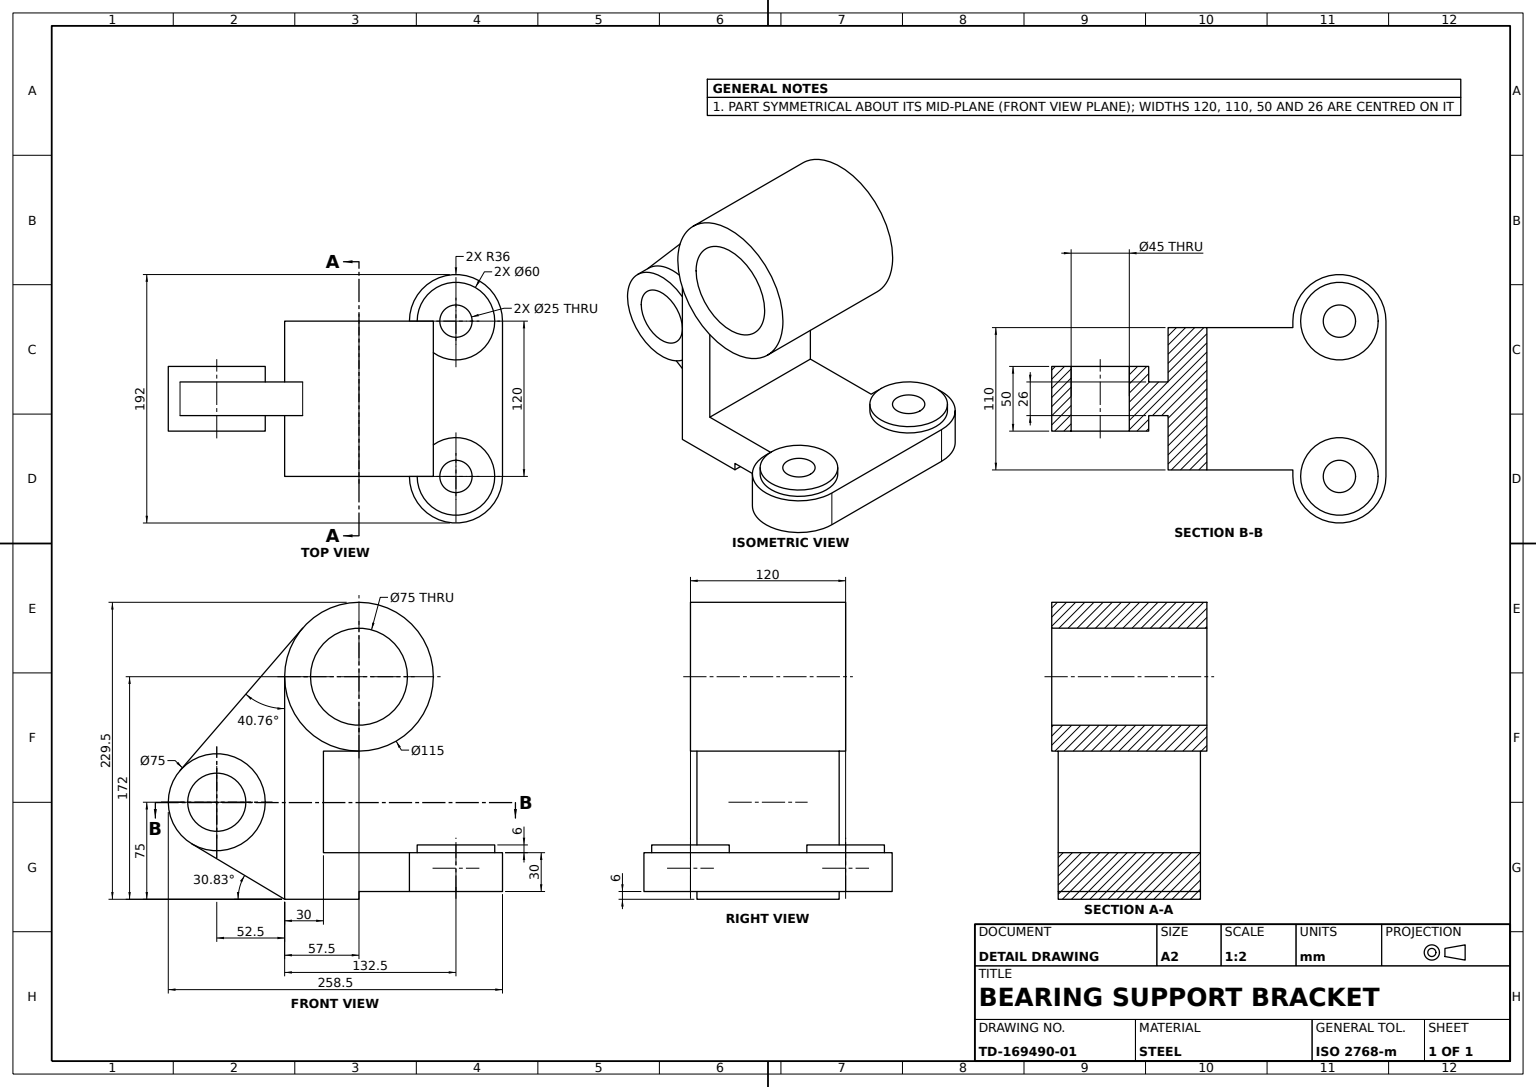
from build123d import *

# Parameters (mm, degrees)
BEARING_HOUSING_SKETCH_R   = 57.5
BEARING_HOUSING_SKETCH_R_2 = 37.5
BEARING_HOUSING_115_DEPTH  = 60
BASE_FOOT_SKETCH_R         = 12.5
BASE_FOOT_DEPTH            = 30
MOUNTING_PAD_SKETCH_R      = 30
MOUNTING_PAD_SKETCH_R_2    = 12.5
MOUNTING_PAD_DEPTH         = 6
SUPPORT_WEB_DEPTH          = 55
SIDE_BOSS_SKETCH_R         = 37.5
SIDE_BOSS_SKETCH_R_2       = 22.5
SIDE_BOSS_75_DEPTH         = 25
GUSSET_RIB_DEPTH           = 13


with BuildPart() as part:
    # Bearing Housing Sketch → Bearing Housing Ø115 (new, symmetric)
    with BuildSketch(Plane(origin=(0, 0, 0), x_dir=(0, 0, -1), z_dir=(1, 0, 0))):
        Circle(BEARING_HOUSING_SKETCH_R)
        Circle(BEARING_HOUSING_SKETCH_R_2, mode=Mode.SUBTRACT)
    extrude(amount=BEARING_HOUSING_115_DEPTH, both=True)



with BuildPart() as body_2:
    # Base Foot Sketch → Base Foot (new body)
    with BuildSketch(Plane(origin=(0, -166, 0), x_dir=(1, 0, 0), z_dir=(0, 1, 0))):
        with BuildLine():
            Line((-60, 111), (60, 111))
            ThreePointArc((60, 111), (96, 75), (60, 39))
            Line((60, 39), (-60, 39))
            ThreePointArc((-60, 39), (-96, 75), (-60, 111))
        make_face()
        with Locations(Location((60, 75, 0), (0, 0, 270))):
            Circle(BASE_FOOT_SKETCH_R, mode=Mode.SUBTRACT)
        with Locations(Location((-60, 75, 0), (0, 0, 270))):
            Circle(BASE_FOOT_SKETCH_R, mode=Mode.SUBTRACT)
    extrude(amount=BASE_FOOT_DEPTH)

    # Mounting Pad Sketch → Mounting Pad (add)
    # profile 1 of 2: a face of its own
    with BuildSketch(Plane(origin=(0, -136, 0), x_dir=(1, 0, 0), z_dir=(0, 1, 0))):
        with Locations(Location((60, 75, 0), (0, 0, 270))):
            Circle(MOUNTING_PAD_SKETCH_R)
        with Locations(Location((60, 75, 0), (0, 0, 270))):
            Circle(MOUNTING_PAD_SKETCH_R_2, mode=Mode.SUBTRACT)
    # profile 2 of 2: a face of its own
    with BuildSketch(Plane(origin=(0, -136, 0), x_dir=(1, 0, 0), z_dir=(0, 1, 0))):
        with Locations(Location((-60, 75, 0), (0, 0, 270))):
            Circle(MOUNTING_PAD_SKETCH_R)
        with Locations(Location((-60, 75, 0), (0, 0, 270))):
            Circle(MOUNTING_PAD_SKETCH_R_2, mode=Mode.SUBTRACT)
    extrude(amount=MOUNTING_PAD_DEPTH)


with BuildPart() as part_1:
    add(part.part)

    add(body_2.part)  # Support Web merges body 2
    # Support Web Sketch → Support Web (add, symmetric)
    with BuildSketch(Plane(origin=(0, 0, 0), x_dir=(0, 0, -1), z_dir=(1, 0, 0))):
        with BuildLine():
            Line((-57.5, 0), (-57.5, -172))
            Line((-57.5, -172), (0, -172))
            Line((0, -172), (0, -166))
            Line((0, -166), (39, -166))
            Line((39, -166), (39, -136))
            Line((39, -136), (-27.5, -136))
            Line((-27.5, -136), (-27.5, -57.5))
            Line((-27.5, -57.5), (0, -57.5))
            ThreePointArc((0, -57.5), (-40.658639918, -40.658639918), (-57.5, 0))
        make_face()
    extrude(amount=SUPPORT_WEB_DEPTH, both=True)



with BuildPart() as body_2_2:
    # Side Boss Sketch → Side Boss Ø75 (new, symmetric)
    with BuildSketch(Plane(origin=(0, 0, 0), x_dir=(0, 0, -1), z_dir=(1, 0, 0))):
        with Locations((-110, -97)):
            Circle(SIDE_BOSS_SKETCH_R)
        with Locations((-110, -97)):
            Circle(SIDE_BOSS_SKETCH_R_2, mode=Mode.SUBTRACT)
    extrude(amount=SIDE_BOSS_75_DEPTH, both=True)


with BuildPart() as part_2:
    add(part_1.part)

    add(body_2_2.part)  # Gusset Rib merges body 2 2
    # Gusset Rib Sketch → Gusset Rib (add, symmetric)
    with BuildSketch(Plane(origin=(0, 0, 0), x_dir=(0, 0, -1), z_dir=(1, 0, 0))):
        with BuildLine():
            Line((-138.406251821, -72.518683502), (-43.556252792, 37.53801863))
            ThreePointArc((-43.556252792, 37.53801863), (-53.901458865, 20.022056144), (-57.5, 0))
            Line((-57.5, 0), (-57.5, -172))
            Line((-57.5, -172), (-129.216934712, -129.201854299))
            ThreePointArc((-129.216934712, -129.201854299), (-72.983281658, -90.998953157), (-138.406251821, -72.518683502))
        make_face()
    extrude(amount=GUSSET_RIB_DEPTH, both=True)


solid = part_2.part
